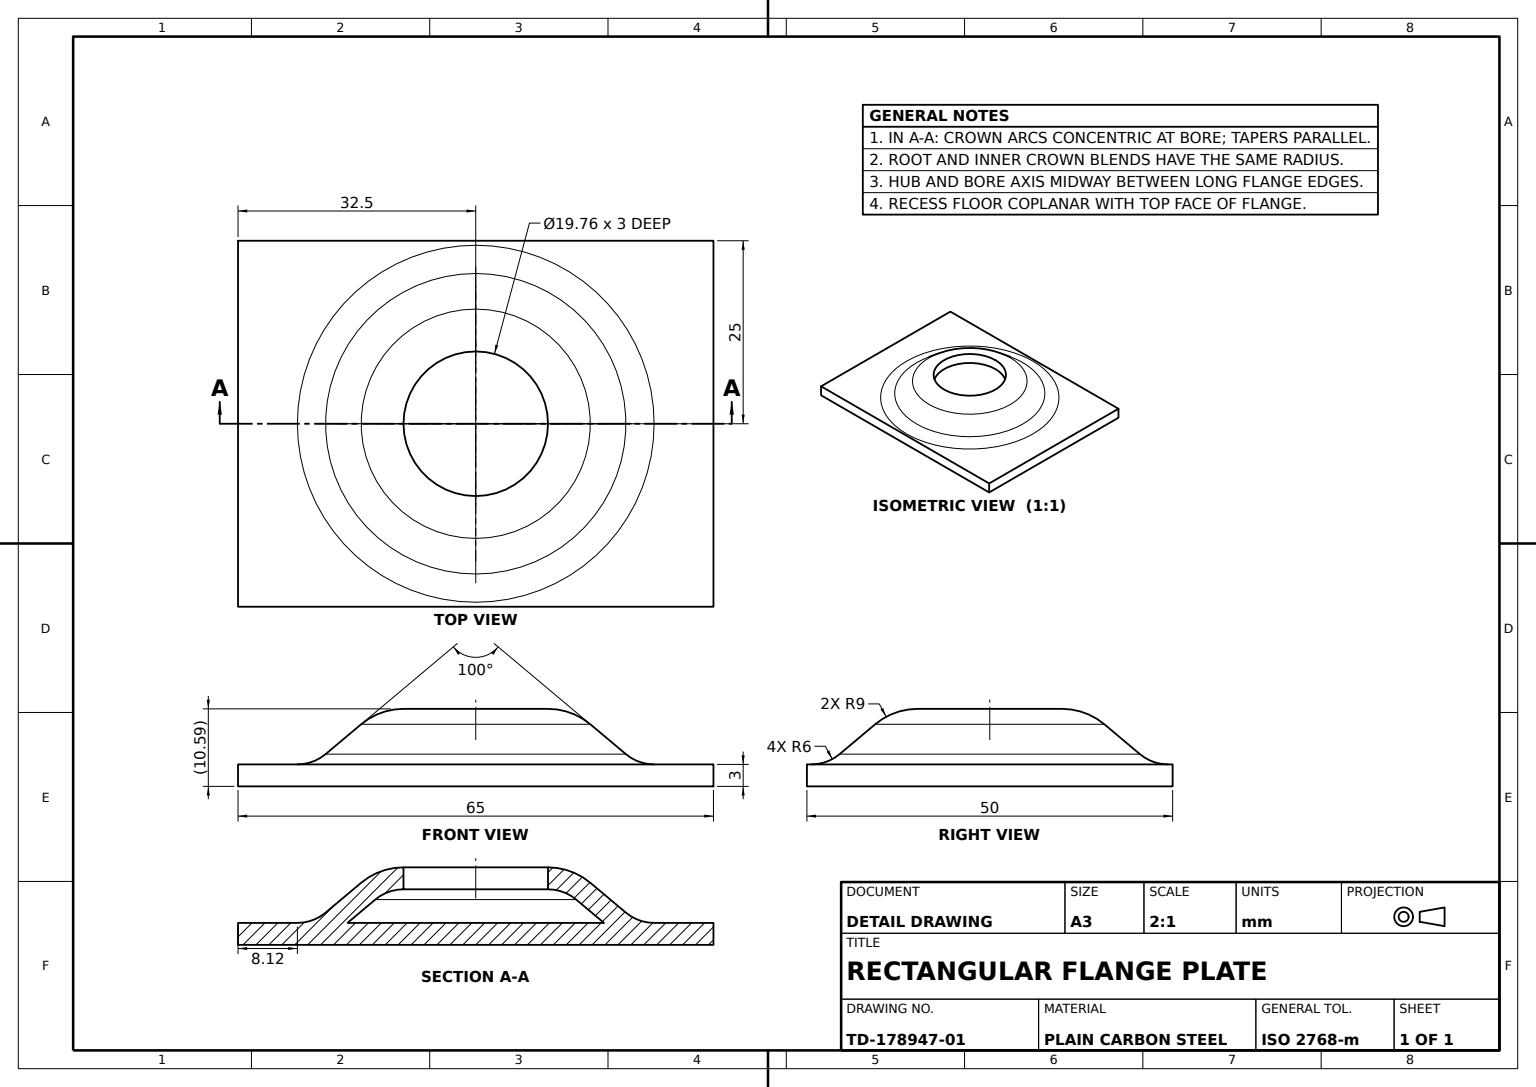
from build123d import *

# Parameters (mm, degrees)
HUB_PROFILE_SKETCH_W                   = 7
HUB_PROFILE_SKETCH_H                   = 3
PLATE_OUTLINE_SKETCH_65X50_OUTSIDE_W   = 85.506
PLATE_OUTLINE_SKETCH_65X50_OUTSIDE_H   = 85.506
PLATE_OUTLINE_SKETCH_65X50_OUTSIDE_W_2 = 65
PLATE_OUTLINE_SKETCH_65X50_OUTSIDE_H_2 = 50
HUB_TRIM_CUT_65X50_DEPTH               = 10
BASE_PLATE_SKETCH_65X50_W              = 65
BASE_PLATE_SKETCH_65X50_H              = 50
BASE_PLATE_65X50X3_DEPTH               = 3
PLATE_CORNER_FILLETS_R6_R              = 6
MOUNTING_HOLES_SKETCH_R                = 2.5
MOUNTING_HOLES_4X_DEPTH                = 3
MOUNTING_HOLE_CHAMFERS_1_5X45_SIZE     = 1.5
CENTER_BORE_SKETCH_R                   = 9.879541092
CENTER_BORE_CUT_DEPTH                  = 23
HUB_GROOVE_SKETCH_45_R                 = 22.5
HUB_GROOVE_45_DEPTH                    = 3
SKETCH3_2_W                            = 65
SKETCH3_2_H                            = 50
PLATE_STEP_65X50X3_DEPTH               = 3


with BuildPart() as part:
    # Hub Profile Sketch → Hub Revolve (revolve)
    with BuildSketch(Plane.XY, mode=Mode.PRIVATE) as hub_revolve_sk:
        with Locations((3.5, 9.089822415)):
            Rectangle(HUB_PROFILE_SKETCH_W, HUB_PROFILE_SKETCH_H)
        with BuildLine():
            Line((9.879541092, 10.589822415), (7, 10.589822415))
            Line((7, 10.589822415), (7, 7.589822415))
            Line((7, 7.589822415), (9.879541092, 7.589822415))
            ThreePointArc((9.879541092, 7.589822415), (11.931661952, 7.22797814), (13.73626675, 6.186089074))
            Line((13.73626675, 6.186089074), (18.599204249, 2.105600012))
            ThreePointArc((18.599204249, 2.105600012), (21.306111446, 0.542766413), (24.384292736, 0))
            Line((24.384292736, 0), (32.5, 0))
            Line((32.5, 0), (32.5, 3))
            Line((32.5, 3), (24.384292736, 3))
            ThreePointArc((24.384292736, 3), (22.332171876, 3.361844275), (20.527567078, 4.403733341))
            Line((20.527567078, 4.403733341), (15.664629579, 8.484222403))
            ThreePointArc((15.664629579, 8.484222403), (12.957722382, 10.047056002), (9.879541092, 10.589822415))
        make_face()
    revolve(hub_revolve_sk.sketch.rotate(Axis((0, 0, 0), (0, 1, 0)), 90), axis=Axis((0, 0, 0), (0, 1, 0)))

    # Plate Outline Sketch 65x50 outside → Hub Trim Cut 65x50 (cut)
    with BuildSketch(Plane(origin=(0, 3, 0), x_dir=(1, 0, 0), z_dir=(0, 1, 0))):
        Rectangle(PLATE_OUTLINE_SKETCH_65X50_OUTSIDE_W, PLATE_OUTLINE_SKETCH_65X50_OUTSIDE_H)
        Rectangle(PLATE_OUTLINE_SKETCH_65X50_OUTSIDE_W_2, PLATE_OUTLINE_SKETCH_65X50_OUTSIDE_H_2, mode=Mode.SUBTRACT)
    extrude(amount=-HUB_TRIM_CUT_65X50_DEPTH, mode=Mode.SUBTRACT)

    # Base Plate Sketch 65x50 → Base Plate 65x50x3 (add)
    with BuildSketch(Plane(origin=(0, 3, 0), x_dir=(1, 0, 0), z_dir=(0, 1, 0))):
        Rectangle(BASE_PLATE_SKETCH_65X50_W, BASE_PLATE_SKETCH_65X50_H)
    extrude(amount=-BASE_PLATE_65X50X3_DEPTH)

    # Plate Corner Fillets R6
    plate_corner_fillets_r6_edges = [part.edges().sort_by_distance(p)[0] for p in [
        (32.5, 1.5, -25),
        (32.5, 1.5, 25),
        (-32.5, 1.5, 25),
        (-32.5, 1.5, -25),
    ]]
    fillet(plate_corner_fillets_r6_edges, radius=PLATE_CORNER_FILLETS_R6_R)

    # Mounting Holes Sketch → Mounting Holes 4x (cut)
    with BuildSketch(Plane(origin=(0, 3, 0), x_dir=(1, 0, 0), z_dir=(0, 1, 0))):
        with Locations(Location((-26.5, 19, 0), (0, 0, 270))):
            Circle(MOUNTING_HOLES_SKETCH_R)
        with Locations(Location((26.5, 19, 0), (0, 0, 270))):
            Circle(MOUNTING_HOLES_SKETCH_R)
        with Locations(Location((26.5, -19, 0), (0, 0, 270))):
            Circle(MOUNTING_HOLES_SKETCH_R)
        with Locations(Location((-26.5, -19, 0), (0, 0, 270))):
            Circle(MOUNTING_HOLES_SKETCH_R)
    extrude(amount=-MOUNTING_HOLES_4X_DEPTH, mode=Mode.SUBTRACT)

    # Mounting Hole Chamfers 1.5x45
    mounting_hole_chamfers_1_5x45_edges = [part.edges().sort_by_distance(p)[0] for p in [
        (-26.5, 3, 16.5),
        (26.5, 3, 16.5),
        (26.5, 3, -21.5),
        (-26.5, 3, -21.5),
    ]]
    chamfer(mounting_hole_chamfers_1_5x45_edges, length=MOUNTING_HOLE_CHAMFERS_1_5X45_SIZE)

    # Center Bore Sketch → Center Bore Cut (cut)
    with BuildSketch(Plane(origin=(0, 10.589822415, 0), x_dir=(1, 0, 0), z_dir=(0, 1, 0))):
        with Locations(Location((0, 0, 0), (0, 0, 90))):
            Circle(CENTER_BORE_SKETCH_R)
    extrude(amount=-CENTER_BORE_CUT_DEPTH, mode=Mode.SUBTRACT)

    # Hub Groove Sketch _45 → Hub Groove _45 (cut)
    with BuildSketch(Plane.XZ):
        with Locations(Location((0, 0, 0), (0, 0, 270))):
            Circle(HUB_GROOVE_SKETCH_45_R)
    extrude(amount=-HUB_GROOVE_45_DEPTH, mode=Mode.SUBTRACT)

    # Sketch3_2 → Plate Step 65x50x3 (add)
    with BuildSketch(Plane(origin=(0, 3, 0), x_dir=(1, 0, 0), z_dir=(0, 1, 0))):
        Rectangle(SKETCH3_2_W, SKETCH3_2_H)
    extrude(amount=-PLATE_STEP_65X50X3_DEPTH)


solid = part.part
